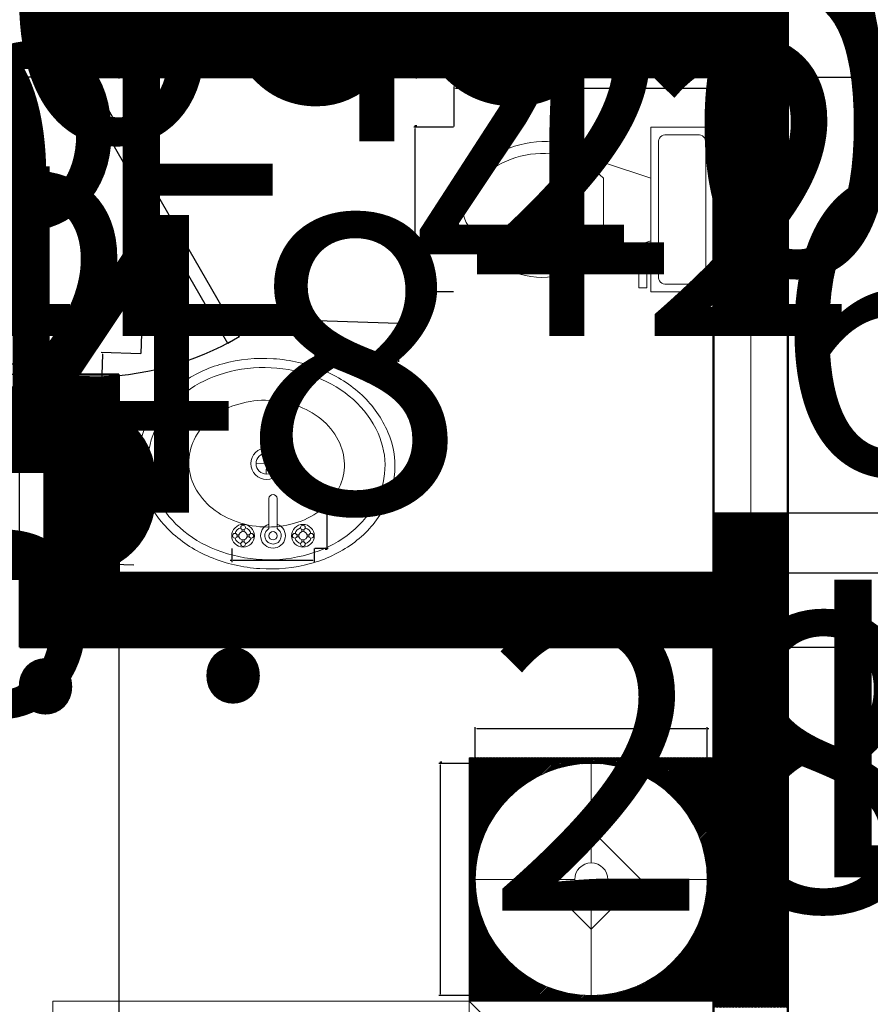
# Model space of a CAD drawing. Units: inches. Extents: x 1173 to 2157, y 515 to 1129.
# Tile 7 of 13: x 1578 to 1681, y 743 to 862. Entities that reach past the tile are written whole.
import ezdxf

# ---------------------------------------------------------------- set-up
doc = ezdxf.new("R2010")
doc.units = ezdxf.units.IN
doc.header["$MEASUREMENT"] = 0
for name, color, linetype, lineweight in [('A-ANNO-DIMS', 2, 'Continuous', 18), ('A-DOOR', 3, 'Continuous', 25), ('A-FLOR-FIXT', 9, 'Continuous', 18), ('A-FURN', 8, 'Continuous', 18), ('A-GLAZ', 4, 'Continuous', 18), ('A-WALL', 7, 'Continuous', 50)]:
    doc.layers.add(name, color=color, linetype=linetype, lineweight=lineweight)
doc.layers.add('A-FURN-PATT', color=7, linetype='Continuous', lineweight=13, true_color=0xffffff)
doc.layers.add('A-WALL-PATT', color=22, linetype='Continuous', lineweight=13, true_color=0xca4b0c)
doc.styles.get("Standard").update_dxf_attribs({"font": 'arial.ttf'})
doc.dimstyles.get("Standard").update_dxf_attribs({"dimtxt": 36, "dimasz": 0.18, "dimexe": 0.18, "dimexo": 0.0625, "dimgap": 0.09, "dimtad": 0, "dimtih": 1, "dimtoh": 1, "dimdec": 0, "dimrnd": 72, "dimzin": 0, "dimdsep": 46, "dimlunit": 3, "dimtxsty": 'Standard', "dimcen": 2, "dimadec": 0, "dimazin": 0, "dimtfac": 1, "dimtdec": 0, "dimtofl": 0, "dimtmove": 0, "dimatfit": 3, "dimfxl": 1, "dimtolj": 1, "dimtzin": 0, "dimarcsym": 0})

# ---------------------------------------------------------------- blocks, each defined once
blk = doc.blocks.new('*U5')
for p, q in [((-40, 0), (-40, 6)), ((0, 0), (0, 6))]:
    blk.add_line(p, q)
blk.add_lwpolyline([(0, 0), (-34.64, -20), (-35.52, -18.48), (-0.88, 1.52)], close=True)
blk.add_arc((0, 0), 40, 180, 210)
blk = doc.blocks.new('Lamp - Table')
for p, q in [((0, 7), (0, 1)), ((0, 3), (-3, 0)), ((3, 0), (0, 3)), ((-1, 0), (-7, 0)), ((-3, 0), (0, -3)), ((0, -3), (3, 0)), ((1, 0), (7, 0)), ((0, -1), (0, -7))]:
    blk.add_line(p, q)
for radius in [7, 1]:
    blk.add_circle((0, 0), radius)
blk = doc.blocks.new('Toilet - top')
for p, q in [((9.5, -6), (9.5, -2)), ((-10, -8.5), (-8, -8.5)), ((-10, -9.5), (-10, -8.5)), ((-8, -8.5), (-8, -8)), ((-7, -8), (-7, -9.5)), ((-4, -8), (-6, -14)), ((4, -8), (6, -14)), ((-7, -9.5), (-10, -9.5)), ((4, -14), (-4, -14))]:
    blk.add_line(p, q)
blk.add_lwpolyline([(10.5, -8), (10.5, 0), (-10.5, 0), (-10.5, -8)], close=True)
for points in [[(8.5, -1), (-8.5, -1)], [(-9.5, -2), (-9.5, -6)], [(-8.5, -7), (8.5, -7)]]:
    blk.add_lwpolyline(points)
for centre, radius, start, end in [((-8.62, -1.88), 0.884, 81.8699, 188.1301), ((8.62, -1.88), 0.884, 351.8699, 98.1301), ((-8.62, -6.12), 0.884, 171.8699, 278.1301), ((8.62, -6.12), 0.884, 261.8699, 8.1301), ((3.52, -21.58), 12.17, 141.4691, 247.9714), ((4.2, -21.82), 11.33, 136.3677, 238.9468), ((-3.52, -21.58), 12.17, 292.0284, 38.5307), ((-4.2, -21.82), 11.33, 301.053, 43.6321), ((0, -27.88), 4, 245.7318, 294.2682), ((0, -29), 4, 254.8605, 285.1395)]:
    blk.add_arc(centre, radius, start, end)
blk = doc.blocks.new('Sink - Oval top')
for p, q in [((0, 1), (0, -1)), ((-1, 0), (1, 0))]:
    blk.add_line(p, q)
for points in [[(-12.234, 0.394, 0.117634), (-11.465, -3.362, 0.104469), (-8.879, -6.804, 0.090016), (-5.083, -9.072, 0.08192), (-0.323, -10.016, 0.08192), (4.488, -9.381, 0.090016), (8.422, -7.361, 0.104469), (11.224, -4.093, 0.117634), (12.234, -0.394, 0.117634), (11.465, 3.362, 0.104469), (8.879, 6.804, 0.090016), (5.083, 9.072, 0.08192), (0.323, 10.016, 0.08192), (-4.488, 9.381, 0.090016), (-8.422, 7.361, 0.104469), (-11.224, 4.093, 0.117634)], [(-11.286, 0.159, 0.118622), (-10.516, -3.253, 0.104678), (-8.072, -6.359, 0.089562), (-4.538, -8.367, 0.081185), (-0.129, -9.152, 0.081185), (4.3, -8.492, 0.089562), (7.889, -6.584, 0.104678), (10.42, -3.548, 0.118622), (11.286, -0.159, 0.118622), (10.516, 3.253, 0.104678), (8.072, 6.359, 0.089562), (4.538, 8.367, 0.081185), (0.129, 9.152, 0.081185), (-4.3, 8.492, 0.089562), (-7.889, 6.584, 0.104678), (-10.42, 3.548, 0.118622)], [(-7.42, 0.083, 0.118283), (-6.907, -2.167, 0.104607), (-5.295, -4.21, 0.089718), (-2.967, -5.528, 0.081436), (-0.068, -6.037, 0.081436), (2.842, -5.593, 0.089718), (5.199, -4.327, 0.104607), (6.857, -2.321, 0.118283), (7.42, -0.083, 0.118283), (6.907, 2.167, 0.104607), (5.295, 4.21, 0.089718), (2.967, 5.528, 0.081436), (0.068, 6.037, 0.081436), (-2.842, 5.593, 0.089718), (-5.199, 4.327, 0.104607), (-6.857, 2.321, 0.118283)]]:
    blk.add_lwpolyline(points, format="xyb", close=True)
for radius in [1.5, 1]:
    blk.add_circle((0, 0), radius)
blk = doc.blocks.new('Faucet - Bathroom top')
for p, q in [((-4.107, 0.125), (-4.375, 0.125)), ((-3.75, 0.4788), (-3.75, 0.75)), ((-3.5, 0.482), (-3.5, 0.75)), ((-3.1461, 0.125), (-2.875, 0.125)), ((3.143, 0.125), (2.875, 0.125)), ((3.5, 0.4788), (3.5, 0.75)), ((3.75, 0.482), (3.75, 0.75)), ((4.1039, 0.125), (4.375, 0.125)), ((-4.1039, -0.125), (-4.375, -0.125)), ((-3.75, -0.4821), (-3.75, -0.75)), ((-3.5, -0.4789), (-3.5, -0.75)), ((-3.143, -0.125), (-2.875, -0.125)), ((-0.5, -0.8639), (-0.5, -4.5)), ((0.5, -4.5), (0.5, -0.8631)), ((3.1461, -0.125), (2.875, -0.125)), ((3.5, -0.4821), (3.5, -0.75)), ((3.75, -0.4789), (3.75, -0.75)), ((4.107, -0.125), (4.375, -0.125))]:
    blk.add_line(p, q)
for centre, radius in [((-3.625, 0), 1.375), ((-3.625, 1), 0.2795), ((3.625, 0), 1.375), ((3.625, 1), 0.2795), ((-4.625, 0), 0.2795), ((-3.625, 0), 0.5), ((-2.625, 0), 0.2795), ((0, 0), 0.5), ((2.625, 0), 0.2795), ((3.625, 0), 0.5), ((4.625, 0), 0.2795), ((-3.625, -1), 0.2795), ((3.625, -1), 0.2795)]:
    blk.add_circle(centre, radius)
for centre, radius, start, end in [((0, 0), 1.5, 289.6514, 250.3603), ((-3.625, 0), 1, 105.2407, 164.2093), ((-3.625, 0), 1, 16.44125, 74.07887), ((0, 0), 1, 300.3431, 239.7554), ((3.625, 0), 1, 106.12, 164.0884), ((3.625, 0), 1, 16.23422, 73.90469), ((-3.625, 0), 1, 196.2342, 253.9047), ((-3.625, 0), 1, 286.12, 344.0884), ((3.625, 0), 1, 196.4413, 254.0789), ((3.625, 0), 1, 285.2407, 344.2093), ((0, -4.5), 0.5, 180, 0)]:
    blk.add_arc(centre, radius, start, end)
blk = doc.blocks.new('Bed - Queen')
for p, q in [((0, -80.00003), (0, 0)), ((0, 0), (59.99999, 0)), ((59.99999, 0), (59.99999, -80.00003)), ((7.99999, -1.2), (28.79998, -1.2)), ((7.99999, -14.4), (7.99999, -1.2)), ((28.79998, -1.2), (28.79998, -14.4)), ((31.19999, -1.2), (51.99999, -1.2)), ((31.19999, -14.4), (31.19999, -1.2)), ((51.99999, -1.2), (51.99999, -16.4)), ((0, -14.4), (44.8, -14.4)), ((59.99999, -29.6), (44.8, -14.4)), ((44.8, -14.4), (44.8, -29.6)), ((51.99999, -16.4), (46.79936, -16.4)), ((44.8, -16.8), (0, -16.8)), ((44.8, -29.6), (59.99999, -29.6)), ((59.99999, -80.00003), (0, -80.00003))]:
    blk.add_line(p, q)
blk = doc.blocks.new('BEDROOM-NIGHTSTAND')
blk.add_lwpolyline([(29.6, 29.48), (0, 29.48), (0, 0), (29.6, 0)], close=True)
blk = doc.blocks.new('*D26')
at = {"layer": 'A-ANNO-DIMS', "color": 0, "lineweight": -2, "transparency": 16777216}
for p, q in [((1577.15, 654.34), (1577.15, 661.66)), ((1577.33, 661.48), (1624.97, 661.48)), ((1625.15, 654.34), (1625.15, 661.66)), ((1625.15, 661.48), (1625.33, 661.48))]:
    blk.add_line(p, q, dxfattribs=at)
at = {"layer": 'A-ANNO-DIMS', "color": 0, "transparency": 16777216}
for points in [[(1577.33, 661.51), (1577.33, 661.45), (1577.15, 661.48)], [(1624.97, 661.51), (1624.97, 661.45), (1625.15, 661.48)]]:
    blk.add_solid(points, dxfattribs=at)
at = {"layer": 'Defpoints', "color": 0, "transparency": 16777216}
for p in [(1625.15, 661.48), (1577.15, 654.28), (1625.15, 654.28)]:
    blk.add_point(p, dxfattribs=at)
at = {"layer": 'A-ANNO-DIMS', "color": 0, "transparency": 16777216, "insert": (1831.09, 661.48), "char_height": 36, "attachment_point": 5}
blk.add_mtext('\\A1;WINDOW 48 TYP.', dxfattribs=at)
blk = doc.blocks.new('*D28')
at = {"layer": 'A-ANNO-DIMS', "color": 0, "lineweight": -2, "transparency": 16777216}
for p, q in [((1581.66, 978.31), (1581.66, 966.19)), ((1661.66, 978.31), (1661.66, 966.19)), ((1581.84, 966.37), (1661.48, 966.37)), ((1661.66, 966.37), (1661.84, 966.37))]:
    blk.add_line(p, q, dxfattribs=at)
at = {"layer": 'A-ANNO-DIMS', "color": 0, "transparency": 16777216}
for points in [[(1581.84, 966.4), (1581.84, 966.34), (1581.66, 966.37)], [(1661.48, 966.4), (1661.48, 966.34), (1661.66, 966.37)]]:
    blk.add_solid(points, dxfattribs=at)
at = {"layer": 'Defpoints', "color": 0, "transparency": 16777216}
for p in [(1581.66, 978.37), (1661.66, 978.37), (1661.66, 966.37)]:
    blk.add_point(p, dxfattribs=at)
at = {"layer": 'A-ANNO-DIMS', "color": 0, "transparency": 16777216, "insert": (1904.61, 966.37), "char_height": 36, "attachment_point": 5}
blk.add_mtext('\\A1;QUEEN BED 80 TYP.', dxfattribs=at)
blk = doc.blocks.new('*D30')
at = {"layer": 'A-ANNO-DIMS', "color": 0, "lineweight": -2, "transparency": 16777216}
for p, q in [((1555.97, 736.03), (1563.78, 736.03)), ((1563.6, 735.85), (1563.6, 729.12)), ((1563.6, 684.97), (1563.6, 691.71)), ((1555.97, 684.79), (1563.78, 684.79))]:
    blk.add_line(p, q, dxfattribs=at)
at = {"layer": 'A-ANNO-DIMS', "color": 0, "transparency": 16777216}
for points in [[(1563.57, 735.85), (1563.63, 735.85), (1563.6, 736.03)], [(1563.57, 684.97), (1563.63, 684.97), (1563.6, 684.79)]]:
    blk.add_solid(points, dxfattribs=at)
at = {"layer": 'Defpoints', "color": 0, "transparency": 16777216}
for p in [(1555.91, 736.03), (1563.6, 736.03), (1555.91, 684.79)]:
    blk.add_point(p, dxfattribs=at)
at = {"layer": 'A-ANNO-DIMS', "color": 0, "transparency": 16777216, "insert": (1563.6, 710.41), "char_height": 36, "attachment_point": 5}
blk.add_mtext('\\A1;DESK 51 TYP.', dxfattribs=at)
blk = doc.blocks.new('*D32')
at = {"layer": 'A-ANNO-DIMS', "color": 0, "lineweight": -2, "transparency": 16777216}
for p, q in [((1632.82, 772.28), (1632.82, 776.62)), ((1633, 776.44), (1660.73, 776.44)), ((1660.91, 772.28), (1660.91, 776.62)), ((1660.91, 776.44), (1661.09, 776.44))]:
    blk.add_line(p, q, dxfattribs=at)
at = {"layer": 'A-ANNO-DIMS', "color": 0, "transparency": 16777216}
for points in [[(1633, 776.47), (1633, 776.41), (1632.82, 776.44)], [(1660.73, 776.47), (1660.73, 776.41), (1660.91, 776.44)]]:
    blk.add_solid(points, dxfattribs=at)
at = {"layer": 'Defpoints', "color": 0, "transparency": 16777216}
for p in [(1660.91, 776.44), (1632.82, 772.22), (1660.91, 772.22)]:
    blk.add_point(p, dxfattribs=at)
at = {"layer": 'A-ANNO-DIMS', "color": 0, "transparency": 16777216, "insert": (1823.46, 776.44), "char_height": 36, "attachment_point": 5}
blk.add_mtext('\\A1;LAMP 28 TYP.', dxfattribs=at)
blk = doc.blocks.new('*D33')
at = {"layer": 'A-ANNO-DIMS', "color": 0, "lineweight": -2, "transparency": 16777216}
for p, q in [((1632.75, 772.22), (1628.42, 772.22)), ((1628.6, 772.22), (1628.6, 772.4)), ((1628.6, 772.4), (1628.78, 772.4)), ((1628.6, 744.31), (1628.6, 772.04)), ((1632.75, 744.13), (1628.42, 744.13))]:
    blk.add_line(p, q, dxfattribs=at)
at = {"layer": 'A-ANNO-DIMS', "color": 0, "transparency": 16777216}
for points in [[(1628.57, 772.04), (1628.63, 772.04), (1628.6, 772.22)], [(1628.57, 744.31), (1628.63, 744.31), (1628.6, 744.13)]]:
    blk.add_solid(points, dxfattribs=at)
at = {"layer": 'Defpoints', "color": 0, "transparency": 16777216}
for p in [(1628.6, 772.22), (1632.82, 772.22), (1632.82, 744.13)]:
    blk.add_point(p, dxfattribs=at)
at = {"layer": 'A-ANNO-DIMS', "color": 0, "transparency": 16777216, "insert": (1716.8, 772.4), "char_height": 36, "attachment_point": 5}
blk.add_mtext('\\A1;28 TYP.', dxfattribs=at)
blk = doc.blocks.new('*D36')
at = {"layer": 'A-ANNO-DIMS', "color": 0, "lineweight": -2, "transparency": 16777216}
for p, q in [((1497.87, 905.02), (1487.37, 905.02)), ((1487.55, 904.84), (1487.55, 889.09)), ((1487.55, 835.93), (1487.55, 851.68)), ((1497.87, 835.75), (1487.37, 835.75))]:
    blk.add_line(p, q, dxfattribs=at)
at = {"layer": 'A-ANNO-DIMS', "color": 0, "transparency": 16777216}
for points in [[(1487.52, 904.84), (1487.58, 904.84), (1487.55, 905.02)], [(1487.52, 835.93), (1487.58, 835.93), (1487.55, 835.75)]]:
    blk.add_solid(points, dxfattribs=at)
at = {"layer": 'Defpoints', "color": 0, "transparency": 16777216}
for p in [(1497.94, 905.02), (1487.55, 835.75), (1497.94, 835.75)]:
    blk.add_point(p, dxfattribs=at)
at = {"layer": 'A-ANNO-DIMS', "color": 0, "transparency": 16777216, "insert": (1487.55, 870.38), "char_height": 36, "attachment_point": 5}
blk.add_mtext('\\A1;DINING SET 69', dxfattribs=at)
blk = doc.blocks.new('*D37')
at = {"layer": 'A-ANNO-DIMS', "color": 0, "lineweight": -2, "transparency": 16777216}
for p, q in [((1497.94, 835.69), (1497.94, 825.18)), ((1539.8, 835.69), (1539.8, 825.18)), ((1498.12, 825.36), (1539.62, 825.36)), ((1539.8, 825.36), (1539.98, 825.36))]:
    blk.add_line(p, q, dxfattribs=at)
at = {"layer": 'A-ANNO-DIMS', "color": 0, "transparency": 16777216}
for points in [[(1498.12, 825.39), (1498.12, 825.33), (1497.94, 825.36)], [(1539.62, 825.39), (1539.62, 825.33), (1539.8, 825.36)]]:
    blk.add_solid(points, dxfattribs=at)
at = {"layer": 'Defpoints', "color": 0, "transparency": 16777216}
for p in [(1497.94, 835.75), (1539.8, 835.75), (1539.8, 825.36)]:
    blk.add_point(p, dxfattribs=at)
at = {"layer": 'A-ANNO-DIMS', "color": 0, "transparency": 16777216, "insert": (1566.4, 825.36), "char_height": 36, "attachment_point": 5}
blk.add_mtext('\\A1;42', dxfattribs=at)
blk = doc.blocks.new('*D38')
at = {"layer": 'A-ANNO-DIMS', "color": 0, "lineweight": -2, "transparency": 16777216}
for p, q in [((1471.69, 862.7), (1478.04, 862.7)), ((1477.86, 862.52), (1477.86, 860.65)), ((1477.86, 821.35), (1477.86, 823.22)), ((1471.69, 821.17), (1478.04, 821.17))]:
    blk.add_line(p, q, dxfattribs=at)
at = {"layer": 'A-ANNO-DIMS', "color": 0, "transparency": 16777216}
for points in [[(1477.83, 862.52), (1477.89, 862.52), (1477.86, 862.7)], [(1477.83, 821.35), (1477.89, 821.35), (1477.86, 821.17)]]:
    blk.add_solid(points, dxfattribs=at)
at = {"layer": 'Defpoints', "color": 0, "transparency": 16777216}
for p in [(1471.63, 862.7), (1477.86, 862.7), (1471.63, 821.17)]:
    blk.add_point(p, dxfattribs=at)
at = {"layer": 'A-ANNO-DIMS', "color": 0, "transparency": 16777216, "insert": (1477.86, 841.93), "char_height": 36, "attachment_point": 5}
blk.add_mtext('\\A1;COFFEE TABLE 42', dxfattribs=at)
blk = doc.blocks.new('*D40')
at = {"layer": 'A-ANNO-DIMS', "color": 0, "lineweight": -2, "transparency": 16777216}
for p, q in [((1422.73, 872.86), (1431.84, 872.86)), ((1431.66, 872.68), (1431.66, 861.58)), ((1431.66, 813.04), (1431.66, 824.15)), ((1422.73, 812.86), (1431.84, 812.86))]:
    blk.add_line(p, q, dxfattribs=at)
at = {"layer": 'A-ANNO-DIMS', "color": 0, "transparency": 16777216}
for points in [[(1431.63, 872.68), (1431.69, 872.68), (1431.66, 872.86)], [(1431.63, 813.04), (1431.69, 813.04), (1431.66, 812.86)]]:
    blk.add_solid(points, dxfattribs=at)
at = {"layer": 'Defpoints', "color": 0, "transparency": 16777216}
for p in [(1422.66, 872.86), (1431.66, 872.86), (1422.66, 812.86)]:
    blk.add_point(p, dxfattribs=at)
at = {"layer": 'A-ANNO-DIMS', "color": 0, "transparency": 16777216, "insert": (1431.66, 842.86), "char_height": 36, "attachment_point": 5}
blk.add_mtext('\\A1;LOVESEAT 60', dxfattribs=at)
blk = doc.blocks.new('*D44')
at = {"layer": 'A-ANNO-DIMS', "color": 0, "lineweight": -2, "transparency": 16777216}
for p, q in [((1630.26, 849.3), (1630.26, 854.13)), ((1630.44, 853.95), (1661.48, 853.95)), ((1661.66, 849.3), (1661.66, 854.13)), ((1661.66, 853.95), (1661.84, 853.95))]:
    blk.add_line(p, q, dxfattribs=at)
at = {"layer": 'A-ANNO-DIMS', "color": 0, "transparency": 16777216}
for points in [[(1630.44, 853.98), (1630.44, 853.92), (1630.26, 853.95)], [(1661.48, 853.98), (1661.48, 853.92), (1661.66, 853.95)]]:
    blk.add_solid(points, dxfattribs=at)
at = {"layer": 'Defpoints', "color": 0, "transparency": 16777216}
for p in [(1661.66, 853.95), (1630.26, 849.24), (1661.66, 849.24)]:
    blk.add_point(p, dxfattribs=at)
at = {"layer": 'A-ANNO-DIMS', "color": 0, "transparency": 16777216, "insert": (1799.17, 853.95), "char_height": 36, "attachment_point": 5}
blk.add_mtext('\\A1;WC 31 TYP.', dxfattribs=at)
blk = doc.blocks.new('*D45')
at = {"layer": 'A-ANNO-DIMS', "color": 0, "lineweight": -2, "transparency": 16777216}
for p, q in [((1630.2, 849.24), (1625.37, 849.24)), ((1625.55, 849.24), (1625.55, 849.42)), ((1625.55, 849.42), (1625.73, 849.42)), ((1625.55, 829.46), (1625.55, 849.06)), ((1630.2, 829.28), (1625.37, 829.28))]:
    blk.add_line(p, q, dxfattribs=at)
at = {"layer": 'A-ANNO-DIMS', "color": 0, "transparency": 16777216}
for points in [[(1625.52, 849.06), (1625.58, 849.06), (1625.55, 849.24)], [(1625.52, 829.46), (1625.58, 829.46), (1625.55, 829.28)]]:
    blk.add_solid(points, dxfattribs=at)
at = {"layer": 'Defpoints', "color": 0, "transparency": 16777216}
for p in [(1625.55, 849.24), (1630.26, 849.24), (1630.26, 829.28)]:
    blk.add_point(p, dxfattribs=at)
at = {"layer": 'A-ANNO-DIMS', "color": 0, "transparency": 16777216, "insert": (1713.74, 849.42), "char_height": 36, "attachment_point": 5}
blk.add_mtext('\\A1;20 TYP.', dxfattribs=at)
blk = doc.blocks.new('*D46')
at = {"layer": 'A-ANNO-DIMS', "color": 0, "lineweight": -2, "transparency": 16777216}
for p, q in [((1646.37, 911.98), (1645.86, 896.32)), ((1648.72, 912.09), (1646.2, 912.17)), ((1648.2, 896.07), (1645.68, 896.15)), ((1645.86, 896.14), (1645.85, 895.96)), ((1645.85, 895.96), (1645.67, 895.96))]:
    blk.add_line(p, q, dxfattribs=at)
at = {"layer": 'A-ANNO-DIMS', "color": 0, "transparency": 16777216}
for points in [[(1646.34, 911.99), (1646.4, 911.98), (1646.38, 912.16)], [(1645.83, 896.32), (1645.89, 896.32), (1645.86, 896.14)]]:
    blk.add_solid(points, dxfattribs=at)
at = {"layer": 'Defpoints', "color": 0, "transparency": 16777216}
for p in [(1648.78, 912.09), (1645.86, 896.14), (1648.26, 896.06)]:
    blk.add_point(p, dxfattribs=at)
at = {"layer": 'A-ANNO-DIMS', "color": 0, "transparency": 16777216, "insert": (1538.16, 895.96), "char_height": 36, "attachment_point": 5}
blk.add_mtext('\\A1;BASIN 16', dxfattribs=at)
blk = doc.blocks.new('*D48')
at = {"layer": 'A-ANNO-DIMS', "color": 0, "lineweight": -2, "transparency": 16777216}
for p, q in [((1592.53, 826.46), (1592.35, 826.47)), ((1592.38, 821.85), (1592.54, 826.64)), ((1623.53, 825.46), (1592.71, 826.46)), ((1623.56, 820.84), (1623.71, 825.64))]:
    blk.add_line(p, q, dxfattribs=at)
at = {"layer": 'A-ANNO-DIMS', "color": 0, "transparency": 16777216}
for points in [[(1592.71, 826.49), (1592.71, 826.43), (1592.53, 826.46)], [(1623.53, 825.49), (1623.53, 825.43), (1623.71, 825.46)]]:
    blk.add_solid(points, dxfattribs=at)
at = {"layer": 'Defpoints', "color": 0, "transparency": 16777216}
for p in [(1592.53, 826.46), (1592.38, 821.79), (1623.56, 820.78)]:
    blk.add_point(p, dxfattribs=at)
at = {"layer": 'A-ANNO-DIMS', "color": 0, "transparency": 16777216, "insert": (1488.3, 826.47), "char_height": 36, "attachment_point": 5}
blk.add_mtext('\\A1;BASIN 31', dxfattribs=at)
blk = doc.blocks.new('*D49')
at = {"layer": 'A-ANNO-DIMS', "color": 0, "lineweight": -2, "transparency": 16777216}
for p, q in [((1587.7, 821.76), (1586.89, 796.55)), ((1592.32, 821.79), (1587.52, 821.94)), ((1586.87, 796.19), (1586.69, 796.19)), ((1591.49, 796.22), (1586.7, 796.37)), ((1586.88, 796.37), (1586.87, 796.19))]:
    blk.add_line(p, q, dxfattribs=at)
at = {"layer": 'A-ANNO-DIMS', "color": 0, "transparency": 16777216}
for points in [[(1587.67, 821.76), (1587.73, 821.76), (1587.7, 821.94)], [(1586.86, 796.55), (1586.92, 796.54), (1586.88, 796.37)]]:
    blk.add_solid(points, dxfattribs=at)
at = {"layer": 'Defpoints', "color": 0, "transparency": 16777216}
for p in [(1592.38, 821.79), (1586.88, 796.37), (1591.56, 796.22)]:
    blk.add_point(p, dxfattribs=at)
at = {"layer": 'A-ANNO-DIMS', "color": 0, "transparency": 16777216, "insert": (1560.52, 796.19), "char_height": 36, "attachment_point": 5}
blk.add_mtext('\\A1;26', dxfattribs=at)
blk = doc.blocks.new('*D50')
at = {"layer": 'A-ANNO-DIMS', "color": 0, "lineweight": -2, "transparency": 16777216}
for p, q in [((1603.33, 798.21), (1603.33, 796.59)), ((1613.33, 798.21), (1613.33, 796.59)), ((1603.33, 796.77), (1603.15, 796.77)), ((1613.15, 796.77), (1603.51, 796.77))]:
    blk.add_line(p, q, dxfattribs=at)
at = {"layer": 'A-ANNO-DIMS', "color": 0, "transparency": 16777216}
for points in [[(1603.51, 796.8), (1603.51, 796.74), (1603.33, 796.77)], [(1613.15, 796.8), (1613.15, 796.74), (1613.33, 796.77)]]:
    blk.add_solid(points, dxfattribs=at)
at = {"layer": 'Defpoints', "color": 0, "transparency": 16777216}
for p in [(1603.33, 798.27), (1613.33, 798.27), (1603.33, 796.77)]:
    blk.add_point(p, dxfattribs=at)
at = {"layer": 'A-ANNO-DIMS', "color": 0, "transparency": 16777216, "insert": (1377.9, 796.77), "char_height": 36, "attachment_point": 5}
blk.add_mtext('\\A1;BASIN TAP 10 TYP.', dxfattribs=at)
blk = doc.blocks.new('*D51')
at = {"layer": 'A-ANNO-DIMS', "color": 0, "lineweight": -2, "transparency": 16777216}
for p, q in [((1613.4, 804.77), (1615.01, 804.77)), ((1614.83, 804.59), (1614.83, 798.45)), ((1613.4, 798.27), (1615.01, 798.27)), ((1614.83, 798.09), (1614.65, 798.09)), ((1614.83, 798.27), (1614.83, 798.09))]:
    blk.add_line(p, q, dxfattribs=at)
at = {"layer": 'A-ANNO-DIMS', "color": 0, "transparency": 16777216}
for points in [[(1614.8, 804.59), (1614.86, 804.59), (1614.83, 804.77)], [(1614.8, 798.45), (1614.86, 798.45), (1614.83, 798.27)]]:
    blk.add_solid(points, dxfattribs=at)
at = {"layer": 'Defpoints', "color": 0, "transparency": 16777216}
for p in [(1613.33, 804.77), (1613.33, 798.27), (1614.83, 798.27)]:
    blk.add_point(p, dxfattribs=at)
at = {"layer": 'A-ANNO-DIMS', "color": 0, "transparency": 16777216, "insert": (1541.08, 798.09), "char_height": 36, "attachment_point": 5}
blk.add_mtext('\\A1;7 TYP.', dxfattribs=at)
blk = doc.blocks.new('*D52')
at = {"layer": 'A-ANNO-DIMS', "color": 0, "lineweight": -2, "transparency": 16777216}
for p, q in [((1589.6, 924.28), (1580.48, 924.28)), ((1580.66, 924.1), (1580.66, 912.75)), ((1580.66, 864.46), (1580.66, 875.81)), ((1589.6, 864.28), (1580.48, 864.28))]:
    blk.add_line(p, q, dxfattribs=at)
at = {"layer": 'A-ANNO-DIMS', "color": 0, "transparency": 16777216}
for points in [[(1580.63, 924.1), (1580.69, 924.1), (1580.66, 924.28)], [(1580.63, 864.46), (1580.69, 864.46), (1580.66, 864.28)]]:
    blk.add_solid(points, dxfattribs=at)
at = {"layer": 'Defpoints', "color": 0, "transparency": 16777216}
for p in [(1580.66, 924.28), (1589.66, 924.28), (1589.66, 864.28)]:
    blk.add_point(p, dxfattribs=at)
at = {"layer": 'A-ANNO-DIMS', "color": 0, "transparency": 16777216, "insert": (1580.66, 894.28), "char_height": 36, "attachment_point": 5}
blk.add_mtext('\\A1;TUB 60', dxfattribs=at)
blk = doc.blocks.new('*D53')
at = {"layer": 'A-ANNO-DIMS', "color": 0, "lineweight": -2, "transparency": 16777216}
for p, q in [((1589.66, 864.22), (1589.66, 855.1)), ((1625.66, 864.22), (1625.66, 855.1)), ((1589.66, 855.28), (1589.48, 855.28)), ((1625.48, 855.28), (1589.84, 855.28))]:
    blk.add_line(p, q, dxfattribs=at)
at = {"layer": 'A-ANNO-DIMS', "color": 0, "transparency": 16777216}
for points in [[(1589.84, 855.31), (1589.84, 855.25), (1589.66, 855.28)], [(1625.48, 855.31), (1625.48, 855.25), (1625.66, 855.28)]]:
    blk.add_solid(points, dxfattribs=at)
at = {"layer": 'Defpoints', "color": 0, "transparency": 16777216}
for p in [(1589.66, 864.28), (1625.66, 864.28), (1589.66, 855.28)]:
    blk.add_point(p, dxfattribs=at)
at = {"layer": 'A-ANNO-DIMS', "color": 0, "transparency": 16777216, "insert": (1563.63, 855.28), "char_height": 36, "attachment_point": 5}
blk.add_mtext('\\A1;36', dxfattribs=at)
blk = doc.blocks.new('*D84')
at = {"layer": 'A-ANNO-DIMS', "color": 0, "lineweight": -2, "transparency": 16777216}
for p, q in [((1661.73, 786.28), (1696.15, 786.28)), ((1695.97, 786.1), (1695.97, 738.76)), ((1695.97, 654.46), (1695.97, 701.8)), ((1661.73, 654.28), (1696.15, 654.28))]:
    blk.add_line(p, q, dxfattribs=at)
at = {"layer": 'A-ANNO-DIMS', "color": 0, "transparency": 16777216}
for points in [[(1695.94, 786.1), (1696, 786.1), (1695.97, 786.28)], [(1695.94, 654.46), (1696, 654.46), (1695.97, 654.28)]]:
    blk.add_solid(points, dxfattribs=at)
at = {"layer": 'Defpoints', "color": 0, "transparency": 16777216}
for p in [(1661.66, 786.28), (1661.66, 654.28), (1695.97, 654.28)]:
    blk.add_point(p, dxfattribs=at)
at = {"layer": 'A-ANNO-DIMS', "color": 0, "transparency": 16777216, "insert": (1695.97, 720.28), "char_height": 36, "attachment_point": 5}
blk.add_mtext('\\A1;132', dxfattribs=at)
blk = doc.blocks.new('*D86')
at = {"layer": 'A-ANNO-DIMS', "color": 0, "lineweight": -2, "transparency": 16777216}
for p, q in [((1529.66, 795.34), (1529.66, 820.76)), ((1529.84, 820.58), (1577.48, 820.58)), ((1577.66, 795.34), (1577.66, 820.76)), ((1577.66, 820.58), (1577.84, 820.58))]:
    blk.add_line(p, q, dxfattribs=at)
at = {"layer": 'A-ANNO-DIMS', "color": 0, "transparency": 16777216}
for points in [[(1529.84, 820.61), (1529.84, 820.55), (1529.66, 820.58)], [(1577.48, 820.61), (1577.48, 820.55), (1577.66, 820.58)]]:
    blk.add_solid(points, dxfattribs=at)
at = {"layer": 'Defpoints', "color": 0, "transparency": 16777216}
for p in [(1577.66, 820.58), (1529.66, 795.28), (1577.66, 795.28)]:
    blk.add_point(p, dxfattribs=at)
at = {"layer": 'A-ANNO-DIMS', "color": 0, "transparency": 16777216, "insert": (1604.48, 820.58), "char_height": 36, "attachment_point": 5}
blk.add_mtext('\\A1;48', dxfattribs=at)
blk = doc.blocks.new('*D95')
at = {"layer": 'A-ANNO-DIMS', "color": 0, "lineweight": -2, "transparency": 16777216}
for p, q in [((1589.66, 795.22), (1589.66, 538.8)), ((1661.66, 795.22), (1661.66, 538.8)), ((1589.84, 538.98), (1600.12, 538.98)), ((1661.48, 538.98), (1651.21, 538.98))]:
    blk.add_line(p, q, dxfattribs=at)
at = {"layer": 'A-ANNO-DIMS', "color": 0, "transparency": 16777216}
for points in [[(1589.84, 539.01), (1589.84, 538.95), (1589.66, 538.98)], [(1661.48, 539.01), (1661.48, 538.95), (1661.66, 538.98)]]:
    blk.add_solid(points, dxfattribs=at)
at = {"layer": 'Defpoints', "color": 0, "transparency": 16777216}
for p in [(1589.66, 795.28), (1661.66, 795.28), (1661.66, 538.98)]:
    blk.add_point(p, dxfattribs=at)
at = {"layer": 'A-ANNO-DIMS', "color": 0, "transparency": 16777216, "insert": (1625.66, 538.98), "char_height": 36, "attachment_point": 5}
blk.add_mtext('\\A1;72', dxfattribs=at)
blk = doc.blocks.new('*D96')
at = {"layer": 'A-ANNO-DIMS', "color": 0, "lineweight": -2, "transparency": 16777216}
for p, q in [((1661.73, 855.28), (1696.15, 855.28)), ((1695.97, 855.1), (1695.97, 843.75)), ((1695.97, 795.46), (1695.97, 806.81)), ((1661.73, 795.28), (1696.15, 795.28))]:
    blk.add_line(p, q, dxfattribs=at)
at = {"layer": 'A-ANNO-DIMS', "color": 0, "transparency": 16777216}
for points in [[(1695.94, 855.1), (1696, 855.1), (1695.97, 855.28)], [(1695.94, 795.46), (1696, 795.46), (1695.97, 795.28)]]:
    blk.add_solid(points, dxfattribs=at)
at = {"layer": 'Defpoints', "color": 0, "transparency": 16777216}
for p in [(1661.66, 855.28), (1695.97, 855.28), (1661.66, 795.28)]:
    blk.add_point(p, dxfattribs=at)
at = {"layer": 'A-ANNO-DIMS', "color": 0, "transparency": 16777216, "insert": (1695.97, 825.28), "char_height": 36, "attachment_point": 5}
blk.add_mtext('\\A1;60', dxfattribs=at)
blk = doc.blocks.new('*D97')
at = {"layer": 'A-ANNO-DIMS', "color": 0, "lineweight": -2, "transparency": 16777216}
for p, q in [((1580.6, 855.28), (1354.18, 855.28)), ((1354.36, 855.28), (1354.36, 855.46)), ((1354.36, 855.46), (1354.54, 855.46)), ((1354.36, 819.46), (1354.36, 855.1)), ((1580.6, 819.28), (1354.18, 819.28))]:
    blk.add_line(p, q, dxfattribs=at)
at = {"layer": 'A-ANNO-DIMS', "color": 0, "transparency": 16777216}
for points in [[(1354.33, 855.1), (1354.39, 855.1), (1354.36, 855.28)], [(1354.33, 819.46), (1354.39, 819.46), (1354.36, 819.28)]]:
    blk.add_solid(points, dxfattribs=at)
at = {"layer": 'Defpoints', "color": 0, "transparency": 16777216}
for p in [(1354.36, 855.28), (1580.66, 855.28), (1580.66, 819.28)]:
    blk.add_point(p, dxfattribs=at)
at = {"layer": 'A-ANNO-DIMS', "color": 0, "transparency": 16777216, "insert": (1380.39, 855.46), "char_height": 36, "attachment_point": 5}
blk.add_mtext('\\A1;36', dxfattribs=at)
blk = doc.blocks.new('*D101')
at = {"layer": 'A-ANNO-DIMS', "color": 0, "lineweight": -2, "transparency": 16777216}
for p, q in [((1670.73, 826.56), (1696.15, 826.56)), ((1695.97, 826.56), (1695.97, 826.74)), ((1695.97, 826.74), (1696.15, 826.74)), ((1695.97, 802.74), (1695.97, 826.38)), ((1670.73, 802.56), (1696.15, 802.56))]:
    blk.add_line(p, q, dxfattribs=at)
at = {"layer": 'A-ANNO-DIMS', "color": 0, "transparency": 16777216}
for points in [[(1695.94, 826.38), (1696, 826.38), (1695.97, 826.56)], [(1695.94, 802.74), (1696, 802.74), (1695.97, 802.56)]]:
    blk.add_solid(points, dxfattribs=at)
at = {"layer": 'Defpoints', "color": 0, "transparency": 16777216}
for p in [(1670.66, 826.56), (1695.97, 826.56), (1670.66, 802.56)]:
    blk.add_point(p, dxfattribs=at)
at = {"layer": 'A-ANNO-DIMS', "color": 0, "transparency": 16777216, "insert": (1722.25, 826.74), "char_height": 36, "attachment_point": 5}
blk.add_mtext('\\A1;24', dxfattribs=at)
blk = doc.blocks.new('*D102')
at = {"layer": 'A-ANNO-DIMS', "color": 0, "lineweight": -2, "transparency": 16777216}
for p, q in [((1661.73, 855.28), (1696.15, 855.28)), ((1695.97, 855.28), (1695.97, 855.46)), ((1695.97, 855.46), (1696.15, 855.46)), ((1695.97, 826.74), (1695.97, 855.1)), ((1670.73, 826.56), (1696.15, 826.56))]:
    blk.add_line(p, q, dxfattribs=at)
at = {"layer": 'A-ANNO-DIMS', "color": 0, "transparency": 16777216}
for points in [[(1695.94, 855.1), (1696, 855.1), (1695.97, 855.28)], [(1695.94, 826.74), (1696, 826.74), (1695.97, 826.56)]]:
    blk.add_solid(points, dxfattribs=at)
at = {"layer": 'Defpoints', "color": 0, "transparency": 16777216}
for p in [(1661.66, 855.28), (1695.97, 855.28), (1670.66, 826.56)]:
    blk.add_point(p, dxfattribs=at)
at = {"layer": 'A-ANNO-DIMS', "color": 0, "transparency": 16777216, "insert": (1757.1, 855.46), "char_height": 36, "attachment_point": 5}
blk.add_mtext('\\A1;28.72', dxfattribs=at)
blk = doc.blocks.new('*D108')
at = {"layer": 'A-ANNO-DIMS', "color": 0, "lineweight": -2, "transparency": 16777216}
for p, q in [((1641.43, 881.4), (1641.43, 885.4)), ((1639.43, 883.4), (1643.43, 883.4)), ((1636.72, 865.51), (1638.44, 872.04)), ((1636.54, 865.51), (1636.72, 865.51))]:
    blk.add_line(p, q, dxfattribs=at)
at = {"layer": 'A-ANNO-DIMS', "color": 0, "transparency": 16777216}
blk.add_solid([(1638.41, 872.05), (1638.47, 872.04), (1638.49, 872.22)], dxfattribs=at)
at = {"layer": 'Defpoints', "color": 0, "transparency": 16777216}
for p in [(1641.43, 883.4), (1638.49, 872.22)]:
    blk.add_point(p, dxfattribs=at)
at = {"layer": 'A-ANNO-DIMS', "color": 0, "transparency": 16777216, "insert": (1505.59, 865.51), "char_height": 36, "attachment_point": 5}
blk.add_mtext('\\A1;2X R11.564', dxfattribs=at)
blk = doc.blocks.new('*D109')
at = {"layer": 'A-ANNO-DIMS', "color": 0, "lineweight": -2, "transparency": 16777216}
for p, q in [((1638.72, 893.14), (1638.9, 893.14)), ((1638.9, 893.14), (1639.74, 886.91)), ((1641.2, 874.07), (1641.2, 878.07)), ((1639.2, 876.07), (1643.2, 876.07))]:
    blk.add_line(p, q, dxfattribs=at)
at = {"layer": 'A-ANNO-DIMS', "color": 0, "transparency": 16777216}
blk.add_solid([(1639.77, 886.92), (1639.71, 886.91), (1639.77, 886.74)], dxfattribs=at)
at = {"layer": 'Defpoints', "color": 0, "transparency": 16777216}
for p in [(1639.77, 886.74), (1641.2, 876.07)]:
    blk.add_point(p, dxfattribs=at)
at = {"layer": 'A-ANNO-DIMS', "color": 0, "transparency": 16777216, "insert": (1507.71, 893.14), "char_height": 36, "attachment_point": 5}
blk.add_mtext('\\A1;2X R10.766', dxfattribs=at)

msp = doc.modelspace()

# ---------------------------------------------------------------- hatches: boundary and pattern name
at = {"layer": 'A-FURN-PATT'}
h = msp.add_hatch(dxfattribs=at)
h.set_pattern_fill('ANSI31', color=256)
h.paths.add_polyline_path([(1661.6635, 772.9167), (1632.0635, 772.9167), (1632.0635, 743.432), (1661.6635, 743.432)])
h.paths.add_polyline_path([(1632.8165, 758.1744, -1), (1660.9104, 758.1744, -1)], flags=16)
h.paths.add_polyline_path([(1646.8635, 752.1542), (1640.8433, 758.1744), (1646.8635, 764.1945), (1652.8836, 758.1744)], flags=0)
h.paths.add_polyline_path([(1644.8567, 758.1744, -1), (1648.8702, 758.1744, -1)], flags=0)
at = {"layer": 'A-WALL-PATT'}
h = msp.add_hatch(dxfattribs=at)
h.set_pattern_fill('ANSI31', color=256)
h.paths.add_polyline_path([(1388.6635, 933.2805), (1388.6635, 1044.2805), (1413.7618, 1044.2805), (1413.7618, 1053.2805), (1379.6635, 1053.2805), (1379.6635, 894.1606), (1388.6635, 894.1606), (1388.6635, 924.2805), (1472.6635, 924.2805), (1472.6635, 933.2805)])
h.paths.add_polyline_path([(1520.6635, 1044.2805), (1520.6635, 1014.7866), (1520.6635, 1005.1794), (1520.7714, 1005.1794), (1520.7714, 956.4707), (1520.6635, 924.2805), (1529.6635, 924.2805), (1529.6635, 931.4788), (1529.6635, 1044.2805), (1530.8474, 1044.2805), (1570.9543, 1044.2805), (1570.9543, 1053.2805), (1461.7618, 1053.2805), (1461.7618, 1044.2805)])
h.paths.add_polyline_path([(1618.9543, 1053.2805), (1618.9543, 1044.2805), (1661.6635, 1044.2805), (1661.6635, 1043.7367), (1661.6635, 1032.8874), (1670.6635, 1032.8874), (1670.6635, 1053.2805)])
h.paths.add_polyline_path([(1661.6635, 933.2805), (1661.6635, 927.8377), (1661.6635, 924.2805), (1661.6635, 918.9156), (1670.6635, 918.9156), (1670.6635, 984.8874), (1661.6635, 984.8874), (1661.6635, 978.3712)])
h.paths.add_polyline_path([(1670.6635, 894.9156), (1661.6635, 894.9156), (1661.6635, 890.0349), (1661.9328, 890.0349), (1661.9328, 870.079), (1661.6635, 864.2805), (1589.6635, 864.2805), (1589.6635, 924.2805), (1625.553, 924.2805, -0.02455299), (1625.3782, 927.8377), (1625.3782, 933.2805), (1577.6635, 933.2805), (1577.6635, 924.2805), (1580.6635, 924.2805), (1580.6635, 855.2805), (1586.1062, 855.2805), (1589.6635, 855.2805), (1661.6635, 855.2805), (1661.6635, 826.5597), (1670.6635, 826.5597)])
h.paths.add_polyline_path([(1670.6635, 802.5597), (1661.6635, 802.5597), (1661.6635, 795.2805), (1589.6635, 795.2805), (1589.6635, 819.17, -0.02455299), (1586.1062, 818.9952), (1580.6635, 818.9952), (1580.6635, 795.2805), (1577.6635, 795.2805), (1577.6635, 786.2805), (1661.6635, 786.2805), (1661.6635, 778.5597), (1661.6635, 742.6973), (1670.6635, 742.6973)])
h.paths.add_polyline_path([(1661.6635, 654.2805), (1625.1498, 654.2805), (1625.1498, 645.2805), (1661.3656, 645.2805), (1661.6635, 645.2805), (1661.6635, 573.2805), (1520.6635, 573.2805), (1520.6635, 564.2805), (1670.6635, 564.2805), (1670.6635, 694.6973), (1661.6635, 694.6973)])
h.paths.add_polyline_path([(1529.4367, 733.4702, -0.06854064), (1529.6635, 734.2623), (1529.6635, 795.2805), (1520.6635, 795.2805), (1520.6635, 645.2805), (1577.1498, 645.2805), (1577.1498, 654.2805), (1529.6635, 654.2805), (1529.6635, 686.5626, -0.06854064), (1529.4367, 687.3547)])
h.paths.add_polyline_path([(1379.6635, 711.2805), (1388.6635, 711.2805), (1458.7214, 711.2805), (1458.7214, 720.2805), (1410.7214, 720.2805), (1388.6635, 720.2805), (1388.6635, 745.0427), (1379.6635, 745.0427)])
h.paths.add_polyline_path([(1388.6635, 846.1606), (1379.6635, 846.1606), (1379.6635, 793.0427), (1388.6635, 793.0427)])

# ---------------------------------------------------------------- linework, layer by layer
at = {"layer": 'A-GLAZ'}
for p, q in [((1666.1635, 802.5597), (1666.1635, 826.5597)), ((1666.1635, 802.5597), (1661.6635, 802.5597)), ((1661.6635, 802.5597), (1670.6635, 802.5597))]:
    msp.add_line(p, q, dxfattribs=at)
for points in [[(1661.6635, 795.2805), (1661.6635, 826.5597), (1670.6635, 826.5597), (1670.6635, 778.5597)], [(1661.6635, 778.5597), (1661.6635, 786.2805)]]:
    msp.add_lwpolyline(points, dxfattribs=at)
at = {"layer": 'A-WALL'}
for p, q in [((1580.6635, 855.2805), (1580.6635, 924.2805)), ((1589.6635, 855.2805), (1580.6635, 855.2805)), ((1661.6635, 855.2805), (1589.6635, 855.2805)), ((1661.6635, 795.2805), (1661.6635, 855.2805)), ((1580.6635, 795.2805), (1580.6635, 819.2805)), ((1589.6635, 819.2805), (1580.6635, 819.2805)), ((1589.6635, 795.2805), (1589.6635, 819.2805)), ((1577.6635, 786.2805), (1577.6635, 795.2805)), ((1580.6635, 795.2805), (1577.6635, 795.2805)), ((1661.6635, 795.2805), (1589.6635, 795.2805)), ((1661.6635, 786.2805), (1577.6635, 786.2805)), ((1661.6635, 654.2805), (1661.6635, 786.2805))]:
    msp.add_line(p, q, dxfattribs=at)
msp.add_lwpolyline([(1379.6635, 564.2805), (1670.6635, 564.2805), (1670.6635, 1053.2805), (1379.6635, 1053.2805)], close=True, dxfattribs=at)

# ---------------------------------------------------------------- block references
at = {"layer": 'A-DOOR', "xscale": 0.9071317920918195, "yscale": 0.9071317920918195, "zscale": 0.9071317920918195, "rotation": 90}
msp.add_blockref('*U5', (1586.1062, 855.2805), dxfattribs=at)
at = {"layer": 'A-FLOR-FIXT'}
for name, p, xscale, yscale, zscale, rotation in [('Toilet - top', (1661.6635, 839.2629), -0.950285164574055, 0.950285164574055, 0.950285164574055, 270), ('Sink - Oval top', (1607.5566, 808.4983), 1.270527326291776, 1.270527326291776, 1.270527326291776, 178.154469915134)]:
    msp.add_blockref(name, p, dxfattribs=dict(at, xscale=xscale, yscale=yscale, zscale=zscale, rotation=rotation))
at = {"layer": 'A-FLOR-FIXT', "rotation": 180}
msp.add_blockref('Faucet - Bathroom top', (1608.3335, 799.768), dxfattribs=at)
at = {"layer": 'A-FURN'}
msp.add_blockref('BEDROOM-NIGHTSTAND', (1632.0635, 743.432), dxfattribs=at)
at = {"layer": 'A-FURN', "xscale": 2.006708061362473, "yscale": 2.006708061362473, "zscale": 2.006708061362473}
msp.add_blockref('Lamp - Table', (1646.8635, 758.1744), dxfattribs=at)
at = {"layer": 'A-FURN', "xscale": -1, "rotation": 270}
msp.add_blockref('Bed - Queen', (1661.6635, 683.432), dxfattribs=at)

# ---------------------------------------------------------------- dimensions: what is measured, and where the dimension line sits
at = {"layer": 'A-ANNO-DIMS'}
for base, p1, p2, text, picture, middle in [((1661.6635, 966.3712), (1581.6634, 978.3712), (1661.6635, 978.3712), 'QUEEN BED <> TYP.', '*D28', (1904.6142, 966.3712)), ((1661.6635, 853.9514), (1630.2601, 849.2409), (1661.6635, 849.2409), 'WC <> TYP.', '*D44', (1799.1681, 853.9514)), ((1660.9104, 776.4354), (1632.8165, 772.2213), (1660.9104, 772.2213), 'LAMP <> TYP.', '*D32', (1823.4628, 776.4354)), ((1625.1498, 661.4805), (1577.1498, 654.2805), (1625.1498, 654.2805), 'WINDOW <> TYP.', '*D26', (1831.0938, 661.4805))]:
    dim = msp.add_linear_dim(base=base, p1=p1, p2=p2, text=text, dimstyle='Standard', override={"dimdec": 0, "dimlfac": 1, "dimrnd": 0, "dimzin": 0, "dimdsep": 46, "dimlunit": 2}, dxfattribs=at)
    dim.commit()
    dim.dimension.update_dxf_attribs({"geometry": picture, "text_midpoint": middle})
for base, p1, p2, angle, text, picture, middle in [((1487.5464, 835.7486), (1497.9367, 905.017), (1497.9367, 835.7486), 270, 'DINING SET <>', '*D36', (1487.5464, 870.3828)), ((1645.8589, 896.1412), (1648.7786, 912.0868), (1648.2623, 896.0638), 268.15447, 'BASIN <>', '*D46', (1538.1601, 895.9613)), ((1580.6635, 924.2805), (1589.6635, 864.2805), (1589.6635, 924.2805), 90, 'TUB <>', '*D52', (1580.6635, 894.2805)), ((1477.8589, 862.6955), (1471.63, 821.1697), (1471.63, 862.6955), 90, 'COFFEE TABLE <>', '*D38', (1477.8589, 841.9326)), ((1603.3335, 796.7679), (1613.3335, 798.2679), (1603.3335, 798.2679), 180, 'BASIN TAP <> TYP.', '*D50', (1377.9039, 796.7679)), ((1625.5496, 849.2409), (1630.2601, 829.2849), (1630.2601, 849.2409), 90, '<> TYP.', '*D45', (1713.7446, 849.4209)), ((1431.6634, 872.8622), (1422.6634, 812.8621), (1422.6634, 872.8622), 90, 'LOVESEAT <>', '*D40', (1431.6634, 842.8622)), ((1592.531, 826.4624), (1623.5567, 820.7814), (1592.3803, 821.786), 178.15447, 'BASIN <>', '*D48', (1488.3007, 826.4682)), ((1614.8335, 798.2679), (1613.3335, 804.768), (1613.3335, 798.2679), 270, '<> TYP.', '*D51', (1541.0778, 798.0879)), ((1628.6024, 772.2213), (1632.8165, 744.1274), (1632.8165, 772.2213), 90, '<> TYP.', '*D33', (1716.7974, 772.4013)), ((1563.5964, 736.0322), (1555.9105, 684.7928), (1555.9105, 736.0322), 90, 'DESK <> TYP.', '*D30', (1563.5964, 710.4125))]:
    dim = msp.add_linear_dim(base=base, p1=p1, p2=p2, angle=angle, text=text, dimstyle='Standard', override={"dimdec": 0, "dimlfac": 1, "dimrnd": 0, "dimzin": 0, "dimdsep": 46, "dimlunit": 2}, dxfattribs=at)
    dim.commit()
    dim.dimension.update_dxf_attribs({"geometry": picture, "text_midpoint": middle})
for center, mpoint, picture, middle in [((1641.2, 876.0658), (1639.765, 886.7357), '*D109', (1507.7105, 893.1376)), ((1641.4252, 883.4015), (1638.487, 872.2169), '*D108', (1505.5919, 865.5062))]:
    dim = msp.add_radius_dim(center=center, mpoint=mpoint, text='2X <>', dimstyle='Standard', override={"dimdec": 3, "dimlfac": 1, "dimrnd": 0, "dimzin": 0, "dimdsep": 46, "dimlunit": 2}, dxfattribs=at)
    dim.commit()
    dim.dimension.update_dxf_attribs({"geometry": picture, "text_midpoint": middle, "dimtype": 164})
for base, p1, p2, angle, override, picture, middle in [((1354.361, 855.2805), (1580.6635, 819.2805), (1580.6635, 855.2805), 90, {"dimdec": 0, "dimlfac": 1, "dimrnd": 0, "dimzin": 0, "dimdsep": 46, "dimlunit": 2}, '*D97', (1380.3908, 855.4605)), ((1589.6635, 855.2805), (1625.6635, 864.2805), (1589.6635, 864.2805), 180, {"dimdec": 0, "dimlfac": 1, "dimrnd": 0, "dimzin": 0, "dimdsep": 46, "dimlunit": 2}, '*D53', (1563.6336, 855.2805)), ((1695.966, 855.2805), (1670.6635, 826.5597), (1661.6635, 855.2805), 90, {"dimdec": 2, "dimlfac": 1, "dimrnd": 0, "dimzin": 0, "dimdsep": 46, "dimlunit": 2}, '*D102', (1757.0995, 855.4605)), ((1695.966, 855.2805), (1661.6635, 795.2805), (1661.6635, 855.2805), 90, {"dimdec": 0, "dimlfac": 1, "dimrnd": 0, "dimzin": 0, "dimdsep": 46, "dimlunit": 2}, '*D96', (1695.966, 825.2805)), ((1695.966, 826.5597), (1670.6635, 802.5597), (1670.6635, 826.5597), 90, {"dimdec": 0, "dimlfac": 1, "dimrnd": 0, "dimzin": 0, "dimdsep": 46, "dimlunit": 2}, '*D101', (1722.2537, 826.7397)), ((1586.8799, 796.3658), (1592.3803, 821.786), (1591.5564, 796.2151), 268.15447, {"dimdec": 0, "dimlfac": 1, "dimrnd": 0, "dimzin": 0, "dimdsep": 46, "dimlunit": 2}, '*D49', (1560.525, 796.1859)), ((1695.966, 654.2805), (1661.6635, 786.2805), (1661.6635, 654.2805), 90, {"dimdec": 0, "dimlfac": 1, "dimrnd": 0, "dimzin": 0, "dimdsep": 46, "dimlunit": 2}, '*D84', (1695.966, 720.2805))]:
    dim = msp.add_linear_dim(base=base, p1=p1, p2=p2, angle=angle, dimstyle='Standard', override=override, dxfattribs=at)
    dim.commit()
    dim.dimension.update_dxf_attribs({"geometry": picture, "text_midpoint": middle})
for base, p1, p2, picture, middle in [((1539.8022, 825.3583), (1497.9367, 835.7486), (1539.8022, 835.7486), '*D37', (1566.3969, 825.3583)), ((1577.6635, 820.583), (1529.6635, 795.2805), (1577.6635, 795.2805), '*D86', (1604.4792, 820.583)), ((1661.6635, 538.978), (1589.6635, 795.2805), (1661.6635, 795.2805), '*D95', (1625.6635, 538.978))]:
    dim = msp.add_linear_dim(base=base, p1=p1, p2=p2, dimstyle='Standard', override={"dimdec": 0, "dimlfac": 1, "dimrnd": 0, "dimzin": 0, "dimdsep": 46, "dimlunit": 2}, dxfattribs=at)
    dim.commit()
    dim.dimension.update_dxf_attribs({"geometry": picture, "text_midpoint": middle})

doc.saveas('drawing.dxf')
